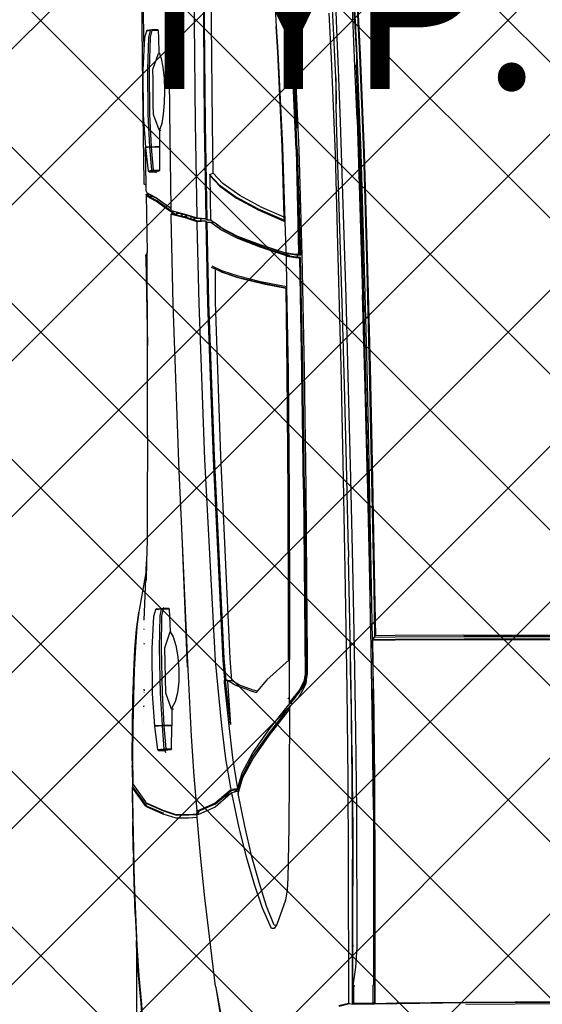
# Model space of a CAD drawing. Units: inches. Extents: x 2167 to 2589, y 1680 to 2489.
# Tile 7 of 38: x 2251 to 2275, y 1727 to 1771. Entities that reach past the tile are written whole.
import ezdxf

# ---------------------------------------------------------------- set-up
doc = ezdxf.new("R2010")
doc.units = ezdxf.units.IN
doc.header["$MEASUREMENT"] = 0
doc.layers.get('0').update_dxf_attribs({"color": 250})
for name, color, linetype, lineweight in [('A-ANNO-DIMS', 2, 'Continuous', 18), ('C-PRKG-VEHS', 8, 'Continuous', 13), ('L-PVMT-PATT', 252, 'Continuous', 13)]:
    doc.layers.add(name, color=color, linetype=linetype, lineweight=lineweight)
doc.layers.add('Edges', color=250, linetype='Continuous')
doc.styles.get("Standard").update_dxf_attribs({"font": 'arial.ttf'})
doc.dimstyles.get("Standard").update_dxf_attribs({"dimtxt": 7, "dimasz": 0.18, "dimexe": 0.18, "dimexo": 0.0625, "dimgap": 0.09, "dimtad": 0, "dimtih": 1, "dimtoh": 1, "dimdec": 1, "dimzin": 0, "dimdsep": 46, "dimlunit": 3, "dimtxsty": 'Standard', "dimcen": 0.09, "dimadec": 0, "dimazin": 0, "dimtfac": 1, "dimtdec": 1, "dimtofl": 0, "dimtmove": 0, "dimatfit": 3, "dimfxl": 1, "dimtolj": 1, "dimtzin": 0, "dimarcsym": 0})

# ---------------------------------------------------------------- blocks, each defined once
blk = doc.blocks.new('Nissan Qashqai pl')
at = {"layer": 'Edges'}
for p, q in [((10.4706, 11.5566), (10.4706, 12.2875)), ((10.4726, 11.5567), (10.4726, 12.2875)), ((10.4764, 11.5569), (10.4764, 12.2872)), ((10.4776, 11.5567), (10.4776, 12.2874)), ((11.056, 11.559), (11.0551, 11.7239)), ((11.0566, 11.5593), (11.0557, 11.724)), ((11.0586, 11.7244), (11.0595, 11.5599)), ((10.4706, 11.5566), (10.4711, 11.4469)), ((10.4731, 11.4469), (10.4726, 11.5567)), ((10.4769, 11.4474), (10.4764, 11.5569)), ((10.4781, 11.4469), (10.4776, 11.5567)), ((11.0572, 11.4499), (11.056, 11.559)), ((11.0579, 11.4504), (11.0566, 11.5593)), ((10.4711, 11.4469), (10.4715, 11.416)), ((10.4735, 11.414), (10.4731, 11.4469)), ((10.4773, 11.4146), (10.4769, 11.4474)), ((10.4785, 11.4111), (10.4781, 11.4469)), ((11.0579, 11.4146), (11.0572, 11.4499)), ((11.0585, 11.4142), (11.0579, 11.4504)), ((10.0431, 11.4075), (9.8673, 11.4031)), ((9.8673, 11.4012), (10.043, 11.4055)), ((10.2215, 11.406), (10.0429, 11.4021)), ((10.2216, 11.4037), (10.0429, 11.3998)), ((10.043, 11.4055), (10.2218, 11.4094)), ((10.2218, 11.4114), (10.0431, 11.4075)), ((10.3564, 11.406), (10.2175, 11.4028)), ((10.3945, 11.4094), (10.2215, 11.406)), ((10.3947, 11.4071), (10.2216, 11.4037)), ((10.3947, 11.4148), (10.2218, 11.4114)), ((10.2218, 11.4094), (10.3947, 11.4128)), ((10.4416, 11.4077), (10.3564, 11.406)), ((10.4773, 11.4107), (10.3945, 11.4094)), ((10.4715, 11.416), (10.3947, 11.4148)), ((10.3947, 11.4128), (10.4735, 11.414)), ((10.4416, 11.4078), (10.3947, 11.4071)), ((10.4519, 11.4079), (10.4416, 11.4077)), ((10.4519, 11.4079), (10.4416, 11.4078)), ((10.4416, 11.4077), (10.4416, 11.4078)), ((10.4524, 11.408), (10.4519, 11.4079)), ((10.4519, 11.4079), (10.4519, 11.4079)), ((10.4524, 11.4079), (10.4519, 11.4079)), ((10.4524, 11.4079), (10.4524, 11.408)), ((10.4533, 11.408), (10.4524, 11.408)), ((10.4533, 11.4079), (10.4524, 11.4079)), ((10.4638, 11.4081), (10.4533, 11.4079)), ((10.4638, 11.4081), (10.4533, 11.408)), ((10.4533, 11.4079), (10.4533, 11.408)), ((10.4914, 11.4087), (10.4638, 11.4081)), ((10.4773, 11.4107), (10.4735, 11.414)), ((10.4773, 11.4146), (10.4773, 11.4107)), ((10.4773, 11.4107), (10.5561, 11.4119)), ((10.4773, 11.4107), (10.4785, 11.4111)), ((10.5563, 11.4123), (10.4785, 11.4111)), ((10.6223, 11.4109), (10.4914, 11.4087)), ((10.6996, 11.4134), (10.5561, 11.4119)), ((10.5563, 11.4123), (10.6999, 11.4138)), ((10.7493, 11.4125), (10.6223, 11.4109)), ((10.7722, 11.4138), (10.6996, 11.4134)), ((10.6999, 11.4138), (10.7722, 11.4142)), ((10.7493, 11.4125), (11.0294, 11.4126)), ((10.7722, 11.4142), (10.7889, 11.4143)), ((10.7722, 11.4142), (10.7722, 11.4138)), ((10.7889, 11.4139), (10.7722, 11.4138)), ((10.7889, 11.4139), (10.7889, 11.4143)), ((10.7889, 11.4143), (10.7923, 11.4143)), ((10.7923, 11.4139), (10.7889, 11.4139)), ((10.7923, 11.4139), (10.7923, 11.4143)), ((10.7923, 11.4143), (10.7933, 11.4143)), ((10.7933, 11.4139), (10.7923, 11.4139)), ((10.7933, 11.4143), (10.827, 11.4145)), ((10.7933, 11.4139), (10.7933, 11.4143)), ((10.8267, 11.4141), (10.7933, 11.4139)), ((10.8267, 11.4141), (11.0585, 11.4142)), ((10.827, 11.4145), (11.0579, 11.4146)), ((11.0294, 11.4118), (11.0281, 11.4118)), ((11.0294, 11.4125), (11.0294, 11.4126)), ((11.0295, 11.4116), (11.0294, 11.4118)), ((11.0568, 11.4118), (11.0294, 11.4118)), ((11.0585, 11.4142), (11.0568, 11.4118)), ((11.0574, 11.3804), (11.0568, 11.4118)), ((11.0585, 11.4142), (11.0579, 11.4146)), ((11.0592, 11.3789), (11.0585, 11.4142)), ((9.5443, 11.3919), (9.4706, 11.388)), ((9.4709, 11.3861), (9.5446, 11.39)), ((9.701, 11.3983), (9.5443, 11.3919)), ((9.5446, 11.39), (9.7011, 11.3963)), ((9.7014, 11.3929), (9.5454, 11.3866)), ((9.7014, 11.3906), (9.5695, 11.3853)), ((9.6472, 11.3861), (9.9278, 11.3949)), ((9.6714, 11.3874), (9.8565, 11.3931)), ((9.8673, 11.4031), (9.701, 11.3983)), ((9.7011, 11.3963), (9.8673, 11.4012)), ((9.8673, 11.3977), (9.7014, 11.3929)), ((9.8673, 11.3954), (9.7014, 11.3906)), ((9.8565, 11.3931), (9.9794, 11.3967)), ((10.0429, 11.4021), (9.8673, 11.3977)), ((10.0429, 11.3998), (9.8673, 11.3954)), ((10.0747, 11.3991), (9.9278, 11.3949)), ((9.9794, 11.3967), (10.0965, 11.3998)), ((10.2043, 11.4025), (10.0747, 11.3991)), ((10.0965, 11.3998), (10.0998, 11.3999)), ((10.0998, 11.3999), (10.2043, 11.4025)), ((10.2175, 11.4028), (10.2043, 11.4025)), ((9.5105, 11.3805), (9.4694, 11.3788)), ((9.5454, 11.3866), (9.472, 11.3828)), ((9.472, 11.3812), (9.5454, 11.3851)), ((9.5755, 11.3834), (9.5105, 11.3805)), ((9.5454, 11.3851), (9.5695, 11.3853)), ((9.5454, 11.3848), (9.5454, 11.3851)), ((9.5695, 11.3853), (9.5609, 11.3849)), ((9.5695, 11.3853), (9.5786, 11.3853)), ((9.6472, 11.3861), (9.5755, 11.3834)), ((9.5786, 11.3853), (9.6206, 11.3861)), ((9.6206, 11.3861), (9.6714, 11.3874)), ((9.9312, 11.3681), (10.0776, 11.3722)), ((10.0776, 11.3722), (10.2201, 11.3759)), ((10.2201, 11.3759), (10.3586, 11.3791)), ((10.3353, 11.3725), (10.2203, 11.3699)), ((10.3353, 11.3725), (10.346, 11.3727)), ((10.4477, 11.3747), (10.346, 11.3727)), ((10.3586, 11.3791), (10.4931, 11.3817)), ((10.4537, 11.3749), (10.4477, 11.3747)), ((10.4537, 11.3749), (10.4538, 11.3749)), ((10.4681, 11.3752), (10.4538, 11.3749)), ((10.4676, 11.3751), (10.4538, 11.3749)), ((10.5576, 11.3766), (10.4676, 11.3751)), ((10.5566, 11.3765), (10.4676, 11.3751)), ((10.4676, 11.3751), (10.4676, 11.3751)), ((10.5866, 11.3772), (10.4681, 11.3752)), ((10.4931, 11.3817), (10.6237, 11.3839)), ((10.5566, 11.3765), (10.7, 11.378)), ((10.6649, 11.3783), (10.5576, 11.3766)), ((10.6649, 11.3783), (10.5866, 11.3772)), ((10.6237, 11.3839), (10.7502, 11.3855)), ((10.6908, 11.3785), (10.6649, 11.3783)), ((10.6649, 11.3783), (10.6772, 11.3784)), ((10.6966, 11.3787), (10.6772, 11.3784)), ((10.6772, 11.3784), (10.6908, 11.3785)), ((10.6991, 11.3786), (10.6908, 11.3785)), ((10.7144, 11.3788), (10.6966, 11.3787)), ((10.6999, 11.3786), (10.6991, 11.3786)), ((10.6999, 11.3786), (10.7808, 11.3793)), ((10.7144, 11.3788), (10.6999, 11.3786)), ((10.7, 11.378), (10.8279, 11.3787)), ((10.8279, 11.3727), (10.7004, 11.372)), ((10.7239, 11.3789), (10.7144, 11.3788)), ((10.7248, 11.3789), (10.7239, 11.3789)), ((10.7808, 11.3793), (10.7248, 11.3789)), ((10.7502, 11.3855), (10.968, 11.3857)), ((10.7808, 11.3793), (10.8711, 11.3796)), ((10.9431, 11.3796), (10.8279, 11.3787)), ((10.8279, 11.3787), (11.0552, 11.3789)), ((10.9614, 11.3788), (10.8279, 11.3787)), ((11.0544, 11.3728), (10.8279, 11.3727)), ((10.896, 11.3796), (10.8711, 11.3796)), ((10.9097, 11.3796), (10.896, 11.3796)), ((10.9431, 11.3796), (10.9097, 11.3796)), ((10.9478, 11.3796), (10.9431, 11.3796)), ((10.9491, 11.3796), (10.9478, 11.3796)), ((10.9668, 11.3796), (10.9491, 11.3796)), ((10.9614, 11.3788), (10.9668, 11.3796)), ((10.9711, 11.3788), (10.9614, 11.3788)), ((10.9668, 11.3796), (10.967, 11.3796)), ((10.9765, 11.3796), (10.967, 11.3796)), ((10.968, 11.3857), (11, 11.3837)), ((10.9765, 11.3796), (10.9711, 11.3788)), ((10.9766, 11.3788), (10.9711, 11.3788)), ((10.9765, 11.3796), (10.9766, 11.3788)), ((10.9825, 11.3796), (10.9765, 11.3796)), ((11.0592, 11.3789), (10.9766, 11.3788)), ((11.0301, 11.3796), (10.9825, 11.3796)), ((11, 11.3837), (11.0301, 11.3796)), ((11.0287, 11.3804), (11.0301, 11.3804)), ((11.0301, 11.3803), (11.0292, 11.3802)), ((11.03, 11.3822), (11.03, 11.3824)), ((11.0301, 11.3803), (11.0301, 11.3804)), ((11.0301, 11.3804), (11.0554, 11.3804)), ((11.0554, 11.3804), (11.0301, 11.3803)), ((11.0301, 11.3796), (11.0301, 11.3803)), ((11.0575, 11.3728), (11.0544, 11.3728)), ((11.0554, 11.3804), (11.0574, 11.3804)), ((11.0592, 11.3789), (11.0574, 11.3804)), ((11.0582, 11.3742), (11.0575, 11.3728)), ((11.0581, 11.3704), (11.0575, 11.3728)), ((11.0582, 11.3742), (11.0592, 11.3789)), ((11.0624, 11.3576), (11.0582, 11.3742)), ((9.5168, 11.3539), (9.5812, 11.3568)), ((9.5812, 11.3568), (9.6514, 11.3592)), ((9.9583, 11.363), (9.651, 11.3536)), ((9.6514, 11.3592), (9.9312, 11.3681)), ((10.0423, 11.3607), (9.8673, 11.3563)), ((10.091, 11.3666), (9.9583, 11.363)), ((10.2211, 11.3646), (10.0423, 11.3607)), ((10.2191, 11.3699), (10.091, 11.3666)), ((10.2202, 11.3699), (10.2191, 11.3699)), ((10.2202, 11.3699), (10.2203, 11.3699)), ((10.3955, 11.368), (10.2211, 11.3646)), ((10.5572, 11.3704), (10.3955, 11.368)), ((10.7004, 11.372), (10.5572, 11.3704)), ((11.0614, 11.3569), (11.0581, 11.3704)), ((9.514, 11.3492), (9.4605, 11.3465)), ((9.4761, 11.3522), (9.5168, 11.3539)), ((9.5503, 11.3455), (9.4782, 11.3418)), ((9.5811, 11.3522), (9.514, 11.3492)), ((9.7029, 11.3516), (9.5503, 11.3455)), ((9.5811, 11.3522), (9.6231, 11.3531)), ((9.594, 11.3527), (9.5811, 11.3522)), ((9.6231, 11.3531), (9.594, 11.3527)), ((9.651, 11.3536), (9.6231, 11.3531)), ((9.8673, 11.3563), (9.7029, 11.3516)), ((9.6953, 11.2892), (9.863, 11.2944)), ((9.6954, 11.2907), (9.8641, 11.2959)), ((9.696, 11.2932), (9.8644, 11.2982)), ((9.7669, 11.2945), (9.7832, 11.2951)), ((9.8629, 11.2925), (9.863, 11.2944)), ((9.8641, 11.2959), (9.863, 11.2944)), ((9.8638, 11.2934), (9.8641, 11.2959)), ((9.8644, 11.2982), (10.0472, 11.3018)), ((9.8681, 11.2959), (9.8678, 11.2935)), ((10.0476, 11.2996), (9.8681, 11.2959)), ((9.8681, 11.2959), (9.869, 11.2946)), ((9.869, 11.2946), (9.8689, 11.2927)), ((10.0477, 11.2982), (9.869, 11.2946)), ((10.0472, 11.3018), (10.2357, 11.3043)), ((10.2367, 11.3022), (10.0476, 11.2996)), ((10.2369, 11.3008), (10.0477, 11.2982)), ((10.2357, 11.3043), (10.53, 11.3068)), ((10.2367, 11.3022), (10.5351, 11.305)), ((10.2369, 11.3008), (10.5348, 11.3036)), ((10.4153, 11.3058), (10.2954, 11.3046)), ((10.4153, 11.3058), (10.4174, 11.3058)), ((10.4174, 11.3058), (10.4181, 11.3058)), ((10.4181, 11.3058), (10.4182, 11.3058)), ((10.4182, 11.3058), (10.53, 11.3068)), ((10.53, 11.3068), (10.5301, 11.3068)), ((10.5301, 11.3068), (10.5323, 11.3065)), ((10.5323, 11.3065), (10.5419, 11.3051)), ((10.5422, 11.3021), (10.5348, 11.3036)), ((10.5424, 11.3035), (10.5351, 11.305)), ((10.5366, 11.3048), (10.536, 11.305)), ((10.5379, 11.3052), (10.5381, 11.305)), ((10.5419, 11.3051), (10.5463, 11.3031)), ((10.5419, 11.3051), (10.5479, 11.3042)), ((10.5522, 11.2977), (10.5422, 11.3021)), ((10.5472, 11.3014), (10.5424, 11.3035)), ((10.5463, 11.3031), (10.5551, 11.2984)), ((10.5546, 11.2982), (10.5472, 11.3014)), ((10.5479, 11.3042), (10.5589, 11.2991)), ((10.5598, 11.2935), (10.5522, 11.2977)), ((10.5583, 11.296), (10.5546, 11.2982)), ((10.5551, 11.2984), (10.5583, 11.296)), ((10.5612, 11.2944), (10.5583, 11.296)), ((10.5589, 11.2991), (10.57, 11.2925)), ((10.5683, 11.2885), (10.5612, 11.2944)), ((9.5437, 11.2822), (9.4735, 11.2779)), ((9.5438, 11.2836), (9.4736, 11.2793)), ((9.4739, 11.282), (9.5443, 11.2863)), ((9.491, 11.2819), (9.5434, 11.2852)), ((9.6953, 11.2892), (9.5437, 11.2822)), ((9.6954, 11.2907), (9.5438, 11.2836)), ((9.5443, 11.2863), (9.696, 11.2932)), ((9.5717, 11.2865), (9.6618, 11.2907)), ((9.6953, 11.2892), (9.8598, 11.2925)), ((9.8652, 11.2788), (9.8516, 11.2363)), ((9.8629, 11.2925), (9.8598, 11.2925)), ((9.8605, 11.2746), (9.8626, 11.2878)), ((9.8615, 11.2754), (9.8635, 11.2886)), ((9.8626, 11.2878), (9.8627, 11.2909)), ((9.8627, 11.2909), (9.8629, 11.2925)), ((9.8627, 11.2909), (9.8637, 11.291)), ((9.8635, 11.2886), (9.8637, 11.291)), ((9.8637, 11.291), (9.8638, 11.2934)), ((9.8637, 11.291), (9.8643, 11.291)), ((9.8643, 11.291), (9.8677, 11.291)), ((9.8652, 11.2738), (9.8652, 11.2788)), ((9.8675, 11.2887), (9.8655, 11.2754)), ((9.8686, 11.2879), (9.8665, 11.2747)), ((9.8677, 11.291), (9.8675, 11.2887)), ((9.8678, 11.2935), (9.8677, 11.291)), ((9.8689, 11.2927), (9.8686, 11.2879)), ((10.2453, 11.2777), (10.4289, 11.2783)), ((10.4289, 11.2783), (10.5092, 11.2783)), ((10.5099, 11.2768), (10.5092, 11.2783)), ((10.5092, 11.2783), (10.5094, 11.2783)), ((10.5094, 11.2783), (10.51, 11.2776)), ((10.5783, 11.2783), (10.5094, 11.2783)), ((10.5764, 11.28), (10.5598, 11.2935)), ((10.5683, 11.2885), (10.573, 11.285)), ((10.575, 11.2829), (10.5683, 11.2885)), ((10.57, 11.2925), (10.5811, 11.2822)), ((10.573, 11.285), (10.5769, 11.2818)), ((10.5776, 11.2808), (10.575, 11.2829)), ((10.5783, 11.2783), (10.5764, 11.28)), ((10.5796, 11.2787), (10.5776, 11.2808)), ((10.5776, 11.2808), (10.5783, 11.2783)), ((10.5796, 11.2787), (10.5783, 11.2783)), ((10.5796, 11.2824), (10.5796, 11.2787)), ((10.6215, 11.2456), (10.5796, 11.2787)), ((10.5811, 11.2822), (10.5821, 11.2808)), ((10.5811, 11.2822), (10.5834, 11.28)), ((10.5821, 11.2808), (10.5834, 11.2793)), ((10.5825, 11.2806), (10.5834, 11.2793)), ((10.5834, 11.28), (10.5851, 11.2783)), ((10.5834, 11.2793), (10.5835, 11.2793)), ((10.5835, 11.2793), (10.584, 11.2787)), ((10.584, 11.2789), (10.584, 11.2793)), ((10.584, 11.2787), (10.584, 11.2789)), ((10.584, 11.2787), (10.6261, 11.2458)), ((10.584, 11.2787), (10.5851, 11.2783)), ((10.5843, 11.2787), (10.584, 11.2787)), ((10.5847, 11.2787), (10.5843, 11.2787)), ((10.5851, 11.2783), (10.5892, 11.2783)), ((10.6306, 11.2459), (10.5892, 11.2783)), ((10.5892, 11.2783), (10.6988, 11.2779)), ((10.6988, 11.2779), (10.7769, 11.2774)), ((9.5403, 11.26), (9.6913, 11.2674)), ((9.6912, 11.2667), (9.5404, 11.2598)), ((9.8039, 11.27), (9.6912, 11.2667)), ((9.6913, 11.2674), (9.8099, 11.2711)), ((9.8039, 11.27), (9.7884, 11.2343)), ((9.7905, 11.2283), (9.8087, 11.2702)), ((9.7925, 11.2294), (9.8107, 11.2711)), ((9.8087, 11.2702), (9.8039, 11.27)), ((9.8099, 11.2711), (9.8087, 11.2702)), ((9.8099, 11.2711), (9.8107, 11.2711)), ((9.8107, 11.2711), (9.8573, 11.2726)), ((9.8475, 11.2312), (9.8611, 11.2734)), ((9.8652, 11.2738), (9.8516, 11.2313)), ((9.8573, 11.2726), (9.8603, 11.2727)), ((9.8603, 11.2727), (9.8605, 11.2746)), ((9.8611, 11.2734), (9.8603, 11.2727)), ((9.8612, 11.2735), (9.8611, 11.2734)), ((9.8612, 11.2735), (9.8615, 11.2754)), ((9.8655, 11.2754), (9.8652, 11.2738)), ((9.8652, 11.2735), (9.8665, 11.2747)), ((9.8652, 11.2738), (9.8652, 11.2738)), ((9.8652, 11.2738), (9.8652, 11.2735)), ((9.8652, 11.2735), (9.8664, 11.2728)), ((9.8665, 11.2747), (9.8664, 11.2728)), ((9.8664, 11.2728), (9.9149, 11.2736)), ((9.9149, 11.2736), (9.9066, 11.2322)), ((9.9169, 11.2728), (9.9086, 11.2313)), ((9.9177, 11.2728), (9.9106, 11.2373)), ((9.9149, 11.2736), (10.0505, 11.276)), ((9.9177, 11.2728), (9.9169, 11.2728)), ((10.0501, 11.2747), (9.9177, 11.2728)), ((10.2453, 11.2762), (10.0501, 11.2747)), ((10.0505, 11.276), (10.2453, 11.2777)), ((10.4292, 11.2767), (10.2453, 11.2762)), ((10.5099, 11.2768), (10.4292, 11.2767)), ((10.51, 11.2776), (10.5099, 11.2768)), ((10.51, 11.2776), (10.5419, 11.2423)), ((10.5705, 11.2771), (10.5709, 11.2767)), ((10.5709, 11.2767), (10.5719, 11.2759)), ((10.7769, 11.2774), (10.858, 11.2759)), ((10.858, 11.2759), (10.8766, 11.2745)), ((10.8766, 11.2745), (10.8932, 11.2722)), ((10.8932, 11.2722), (10.932, 11.258)), ((9.471, 11.2554), (9.4997, 11.2573)), ((9.4997, 11.2573), (9.5403, 11.26)), ((9.5404, 11.2598), (9.4997, 11.2573)), ((10.933, 11.2541), (10.9026, 11.2417)), ((10.9384, 11.2497), (10.9059, 11.2355)), ((10.932, 11.258), (10.9335, 11.257)), ((10.9335, 11.257), (10.933, 11.2541)), ((10.9335, 11.257), (10.9386, 11.2537)), ((10.9386, 11.2537), (10.9384, 11.2497)), ((9.7884, 11.2343), (9.7692, 11.1989)), ((9.8338, 11.1956), (9.8475, 11.2312)), ((9.8516, 11.2363), (9.8378, 11.2007)), ((9.8516, 11.2313), (9.8378, 11.1957)), ((9.9066, 11.2322), (9.8978, 11.197)), ((9.9086, 11.2313), (9.8998, 11.196)), ((9.9106, 11.2373), (9.9018, 11.2021)), ((10.5419, 11.2423), (10.56, 11.2265)), ((10.6583, 11.2197), (10.6215, 11.2456)), ((10.6261, 11.2458), (10.6627, 11.22)), ((10.6671, 11.2203), (10.6306, 11.2459)), ((10.9026, 11.2417), (10.8653, 11.2297)), ((10.9059, 11.2355), (10.8682, 11.2226)), ((9.7713, 11.1929), (9.7905, 11.2283)), ((9.7733, 11.194), (9.7925, 11.2294)), ((10.5584, 11.2206), (10.5502, 11.1986)), ((10.56, 11.2265), (10.5584, 11.2206)), ((10.5584, 11.2136), (10.5617, 11.2251)), ((10.56, 11.2265), (10.5617, 11.2251)), ((10.69, 11.2028), (10.6583, 11.2197)), ((10.6627, 11.22), (10.6943, 11.2032)), ((10.6976, 11.2041), (10.6671, 11.2203)), ((10.8239, 11.2181), (10.7754, 11.2071)), ((10.8653, 11.2297), (10.8239, 11.2181)), ((10.8682, 11.2226), (10.8264, 11.21)), ((9.8378, 11.2007), (9.8241, 11.1736)), ((9.9018, 11.2021), (9.8931, 11.1752)), ((10.5584, 11.2136), (10.5502, 11.1916)), ((10.7155, 11.1952), (10.69, 11.2028)), ((10.6943, 11.2032), (10.7155, 11.1969)), ((10.7228, 11.1965), (10.6976, 11.2041)), ((10.7754, 11.2071), (10.7228, 11.1965)), ((10.8264, 11.21), (10.7776, 11.1982)), ((9.7692, 11.1989), (9.7499, 11.1721)), ((9.7519, 11.1661), (9.7713, 11.1929)), ((9.754, 11.1672), (9.7733, 11.194)), ((9.8201, 11.1685), (9.8338, 11.1956)), ((9.8378, 11.1957), (9.8241, 11.1686)), ((9.8978, 11.197), (9.8891, 11.1701)), ((9.8911, 11.1693), (9.8998, 11.196)), ((10.543, 11.1865), (10.5079, 11.1835)), ((10.5502, 11.1986), (10.543, 11.1865)), ((10.5502, 11.1916), (10.543, 11.1795)), ((10.543, 11.1795), (10.543, 11.1865)), ((10.5439, 11.1796), (10.613, 11.1841)), ((10.613, 11.1841), (10.547, 11.1767)), ((10.6144, 11.1813), (10.6664, 11.1875)), ((10.6664, 11.1875), (10.7155, 11.1952)), ((10.7137, 11.1846), (10.6678, 11.177)), ((10.7165, 11.1851), (10.7137, 11.1846)), ((10.7155, 11.1957), (10.7155, 11.1969)), ((10.7155, 11.1969), (10.7192, 11.1957)), ((10.7209, 11.1902), (10.7155, 11.1957)), ((10.7155, 11.1952), (10.7155, 11.1957)), ((10.7186, 11.1848), (10.7155, 11.1952)), ((10.7155, 11.1952), (10.7165, 11.1851)), ((10.7177, 11.1838), (10.7165, 11.1851)), ((10.7387, 11.1593), (10.7177, 11.1838)), ((10.7312, 11.1701), (10.7186, 11.1848)), ((10.7192, 11.1957), (10.7228, 11.1965)), ((10.7192, 11.1957), (10.7209, 11.1902)), ((10.7209, 11.1902), (10.7221, 11.1861)), ((10.7221, 11.1861), (10.7222, 11.1859)), ((10.7222, 11.186), (10.7221, 11.1861)), ((10.7247, 11.1867), (10.7222, 11.186)), ((10.7222, 11.186), (10.7222, 11.1859)), ((10.7222, 11.1859), (10.7232, 11.1848)), ((10.7222, 11.1859), (10.7224, 11.1855)), ((10.7224, 11.1855), (10.7312, 11.1701)), ((10.7232, 11.1848), (10.7228, 11.1859)), ((10.7232, 11.1848), (10.7449, 11.1598)), ((10.7776, 11.1982), (10.7247, 11.1867)), ((10.7257, 11.1853), (10.7256, 11.1854)), ((11.0357, 11.1613), (11.1598, 11.1847)), ((9.7499, 11.1721), (9.7337, 11.1566)), ((9.8241, 11.1686), (9.8119, 11.1529)), ((9.8241, 11.1736), (9.8147, 11.1616)), ((9.8147, 11.1616), (9.8201, 11.1685)), ((9.8891, 11.1701), (9.8818, 11.1551)), ((9.8911, 11.1691), (9.8867, 11.16)), ((9.8931, 11.1751), (9.8911, 11.1693)), ((9.8911, 11.1693), (9.8911, 11.1691)), ((9.8931, 11.1751), (9.8931, 11.1752)), ((10.1849, 11.1687), (9.9393, 11.1602)), ((10.5079, 11.1835), (10.1849, 11.1687)), ((10.5079, 11.1739), (10.1849, 11.1585)), ((10.1894, 11.1563), (10.5109, 11.1721)), ((10.543, 11.1771), (10.5079, 11.1739)), ((10.5109, 11.1721), (10.5417, 11.1748)), ((10.6152, 11.1702), (10.5113, 11.1603)), ((10.543, 11.1771), (10.5417, 11.1748)), ((10.5417, 11.1748), (10.5427, 11.1739)), ((10.5436, 11.1754), (10.5427, 11.1739)), ((10.5427, 11.1739), (10.5458, 11.1742)), ((10.5439, 11.1796), (10.543, 11.1795)), ((10.543, 11.1795), (10.543, 11.1771)), ((10.544, 11.1763), (10.543, 11.1771)), ((10.544, 11.1763), (10.5436, 11.1754)), ((10.547, 11.1767), (10.544, 11.1763)), ((10.5458, 11.1742), (10.6144, 11.1813)), ((10.6678, 11.177), (10.6152, 11.1702)), ((10.7397, 11.1602), (10.7312, 11.1701)), ((11.0492, 11.1635), (11.1336, 11.1772)), ((9.4936, 11.1538), (9.3225, 11.1531)), ((9.6552, 11.1554), (9.4936, 11.1538)), ((9.7337, 11.1566), (9.6552, 11.1554)), ((9.7357, 11.1507), (9.7337, 11.1566)), ((9.7357, 11.1507), (9.7519, 11.1661)), ((9.7378, 11.1517), (9.754, 11.1672)), ((9.8078, 11.1528), (9.7378, 11.1517)), ((9.8078, 11.1528), (9.8119, 11.1579)), ((9.8078, 11.1471), (9.8078, 11.1528)), ((9.8147, 11.1616), (9.8119, 11.1579)), ((9.8119, 11.1579), (9.8119, 11.1529)), ((9.8119, 11.1529), (9.8119, 11.1472)), ((9.8147, 11.1616), (9.8147, 11.1616)), ((9.8867, 11.16), (9.8838, 11.1541)), ((9.9393, 11.1602), (9.8867, 11.16)), ((10.1849, 11.1585), (9.9393, 11.1497)), ((9.9411, 11.1475), (10.1894, 11.1563)), ((10.5113, 11.1603), (10.19, 11.1433)), ((10.7501, 11.1327), (10.7387, 11.1593)), ((10.7507, 11.1344), (10.7397, 11.1602)), ((10.7449, 11.1598), (10.7563, 11.1333)), ((11.0304, 11.1603), (10.8896, 11.1434)), ((11.0304, 11.1603), (11.0357, 11.1613)), ((11.0357, 11.1613), (11.0491, 11.1635)), ((11.0492, 11.1635), (11.0491, 11.1635)), ((9.3198, 11.1403), (9.4922, 11.1409)), ((9.4936, 11.1428), (9.3225, 11.1421)), ((9.4922, 11.1409), (9.654, 11.1423)), ((9.6552, 11.1445), (9.4936, 11.1428)), ((9.654, 11.1423), (9.8061, 11.1447)), ((9.8078, 11.1471), (9.6552, 11.1445)), ((9.7357, 11.1507), (9.7378, 11.1517)), ((9.8061, 11.1447), (9.8051, 11.1309)), ((9.8055, 11.1298), (9.8058, 11.1369)), ((9.8058, 11.1369), (9.8061, 11.1447)), ((9.8098, 11.1369), (9.8058, 11.1369)), ((9.8061, 11.1447), (9.8078, 11.1471)), ((9.8098, 11.1369), (9.8096, 11.13)), ((9.8101, 11.1449), (9.8098, 11.1369)), ((9.8101, 11.1449), (9.9411, 11.1475)), ((9.8119, 11.1472), (9.8101, 11.1449)), ((9.8101, 11.1449), (9.8112, 11.1311)), ((9.9393, 11.1497), (9.8119, 11.1472)), ((10.19, 11.1433), (9.9414, 11.1341)), ((10.8218, 11.1365), (10.7615, 11.1311)), ((10.8896, 11.1434), (10.8218, 11.1365)), ((9.4919, 11.1269), (9.3194, 11.1262)), ((9.6538, 11.1284), (9.4919, 11.1269)), ((9.802, 11.1309), (9.6538, 11.1284)), ((9.7992, 11.1133), (9.8044, 11.129)), ((9.803, 11.1212), (9.8014, 11.1176)), ((9.8014, 11.1176), (9.8026, 11.1212)), ((9.8051, 11.1309), (9.802, 11.1309)), ((9.8026, 11.1212), (9.8041, 11.1256)), ((9.803, 11.1212), (9.8026, 11.1212)), ((9.8067, 11.1213), (9.803, 11.1212)), ((9.8041, 11.1256), (9.8045, 11.1268)), ((9.8041, 11.1256), (9.8081, 11.1256)), ((9.8044, 11.129), (9.8051, 11.1309)), ((9.8067, 11.1213), (9.8044, 11.1142)), ((9.8045, 11.1268), (9.8046, 11.1271)), ((9.8045, 11.1268), (9.8085, 11.1268)), ((9.8046, 11.1271), (9.8055, 11.1298)), ((9.8086, 11.1271), (9.8046, 11.1271)), ((9.8106, 11.1292), (9.8054, 11.1135)), ((9.8081, 11.1256), (9.8067, 11.1213)), ((9.8085, 11.1268), (9.8081, 11.1256)), ((9.8086, 11.1271), (9.8085, 11.1268)), ((9.8096, 11.13), (9.8086, 11.1271)), ((9.8112, 11.1311), (9.8106, 11.1292)), ((9.8143, 11.1312), (9.8112, 11.1311)), ((9.9414, 11.1341), (9.8143, 11.1312)), ((10.5147, 11.1156), (10.6318, 11.1213)), ((10.6318, 11.1213), (10.6955, 11.1257)), ((10.6955, 11.1257), (10.7509, 11.1302)), ((10.7507, 11.1309), (10.7501, 11.1327)), ((10.7511, 11.1335), (10.7507, 11.1344)), ((10.7507, 11.1344), (10.7524, 11.1335)), ((10.751, 11.131), (10.7507, 11.1309)), ((10.7509, 11.1302), (10.7507, 11.1309)), ((10.7522, 11.1311), (10.7509, 11.1302)), ((10.7516, 11.131), (10.7509, 11.1302)), ((10.7519, 11.1314), (10.7511, 11.1335)), ((10.7519, 11.1314), (10.7516, 11.131)), ((10.7522, 11.1311), (10.7516, 11.131)), ((10.7526, 11.1318), (10.7519, 11.1314)), ((10.7553, 11.1307), (10.7522, 11.1311)), ((10.7524, 11.1335), (10.7526, 11.1318)), ((10.7524, 11.1335), (10.7556, 11.1319)), ((10.7532, 11.1321), (10.7526, 11.1318)), ((10.7526, 11.1318), (10.7526, 11.1314)), ((10.7556, 11.1319), (10.7532, 11.1321)), ((10.7563, 11.1169), (10.7553, 11.1307)), ((10.7556, 11.1319), (10.7561, 11.1317)), ((10.7563, 11.1319), (10.7561, 11.1319)), ((10.7563, 11.1315), (10.7561, 11.1317)), ((10.7561, 11.1317), (10.7563, 11.1317)), ((10.7563, 11.1333), (10.7569, 11.1317)), ((10.7563, 11.1317), (10.7563, 11.1319)), ((10.7563, 11.1317), (10.7569, 11.1317)), ((10.7569, 11.1316), (10.7563, 11.1317)), ((10.7563, 11.1315), (10.7563, 11.1317)), ((10.7572, 11.1178), (10.7563, 11.1315)), ((10.7573, 11.1307), (10.7563, 11.1315)), ((10.7569, 11.1317), (10.7569, 11.1316)), ((10.7569, 11.1316), (10.7573, 11.1307)), ((10.7604, 11.131), (10.7573, 11.1307)), ((10.7615, 11.1311), (10.7604, 11.131)), ((10.7615, 11.1311), (10.7623, 11.1173)), ((9.7937, 11.0918), (9.7992, 11.1133)), ((9.7987, 11.1053), (9.7977, 11.1033)), ((9.7978, 11.1044), (9.7987, 11.108)), ((9.7987, 11.1053), (9.7978, 11.1044)), ((9.7987, 11.108), (9.8002, 11.1141)), ((9.7992, 11.1065), (9.7987, 11.108)), ((9.7992, 11.1065), (9.7987, 11.1053)), ((9.8027, 11.1078), (9.7992, 11.1065)), ((9.8054, 11.1135), (9.7999, 11.0919)), ((9.8002, 11.1141), (9.8008, 11.1157)), ((9.8027, 11.1078), (9.8003, 11.0983)), ((9.8008, 11.1157), (9.8014, 11.1176)), ((9.8014, 11.1139), (9.8008, 11.1157)), ((9.8043, 11.1139), (9.8014, 11.1139)), ((9.8031, 11.1093), (9.8014, 11.1139)), ((9.8031, 11.1093), (9.8027, 11.1078)), ((9.8043, 11.1139), (9.8031, 11.1093)), ((9.8044, 11.1142), (9.8043, 11.1139)), ((10.2081, 11.1017), (10.312, 11.1064)), ((10.312, 11.1064), (10.5147, 11.1156)), ((10.312, 11.1064), (10.5214, 11.1149)), ((10.7565, 11.0969), (10.7563, 11.1169)), ((10.7575, 11.0979), (10.7572, 11.1178)), ((10.7623, 11.1173), (10.7626, 11.0974)), ((9.7965, 11.0915), (9.7894, 11.0806)), ((9.7931, 11.089), (9.7934, 11.0906)), ((9.7933, 11.0892), (9.7941, 11.0901)), ((9.7934, 11.0906), (9.7937, 11.0918)), ((9.7934, 11.0906), (9.7938, 11.0904)), ((9.7941, 11.0901), (9.7943, 11.0907)), ((9.7964, 11.0988), (9.7943, 11.0907)), ((9.7955, 11.0925), (9.7943, 11.0907)), ((9.7963, 11.0918), (9.7955, 11.0925)), ((9.7992, 11.0966), (9.7963, 11.0918)), ((9.7963, 11.0918), (9.7963, 11.0918)), ((9.7964, 11.0917), (9.7963, 11.0918)), ((9.7964, 11.0988), (9.7973, 11.1023)), ((9.7964, 11.0988), (9.7992, 11.0966)), ((9.7964, 11.0917), (9.7996, 11.0966)), ((9.7964, 11.0917), (9.7964, 11.0917)), ((9.7967, 11.0915), (9.7964, 11.0917)), ((9.7965, 11.0915), (9.7967, 11.0915)), ((9.7983, 11.0901), (9.7965, 11.0915)), ((9.7967, 11.0915), (9.7986, 11.0916)), ((9.7977, 11.0907), (9.7967, 11.0915)), ((9.7973, 11.1023), (9.7977, 11.1042)), ((9.7977, 11.1033), (9.7973, 11.1023)), ((9.7973, 11.1023), (9.7977, 11.1011)), ((9.7977, 11.1042), (9.7978, 11.1044)), ((9.7977, 11.1042), (9.7977, 11.1033)), ((9.7977, 11.1011), (9.7977, 11.0998)), ((9.7977, 11.1011), (9.7985, 11.099)), ((9.7977, 11.0998), (9.7985, 11.099)), ((9.7982, 11.0902), (9.7977, 11.0907)), ((9.7986, 11.0916), (9.7982, 11.0902)), ((9.7983, 11.0901), (9.7982, 11.0902)), ((9.7986, 11.0898), (9.7983, 11.0901)), ((9.7985, 11.099), (9.7989, 11.098)), ((9.7988, 11.0925), (9.7986, 11.0916)), ((9.7986, 11.0898), (9.7993, 11.0891)), ((9.7998, 11.0964), (9.7988, 11.0925)), ((9.7989, 11.098), (9.7998, 11.0976)), ((9.7998, 11.0976), (9.7992, 11.0966)), ((9.7999, 11.0919), (9.7993, 11.0891)), ((9.8002, 11.098), (9.7996, 11.0966)), ((9.8001, 11.0974), (9.7996, 11.0966)), ((9.7996, 11.0966), (9.7998, 11.0964)), ((9.8003, 11.0983), (9.7998, 11.0976)), ((9.8001, 11.0974), (9.7998, 11.0964)), ((9.8002, 11.098), (9.8001, 11.0974)), ((9.8003, 11.0983), (9.8002, 11.098)), ((9.8024, 11.0892), (9.9426, 11.0923)), ((9.9426, 11.0923), (10.2081, 11.1017)), ((10.4653, 11.0881), (10.4652, 11.0897)), ((10.4653, 11.0881), (10.4732, 11.0925)), ((10.4732, 11.0925), (10.4871, 11.0967)), ((10.4871, 11.0967), (10.5048, 11.1002)), ((10.5048, 11.1002), (10.5246, 11.1019)), ((10.5246, 11.1019), (10.5445, 11.1017)), ((10.5445, 11.1017), (10.5625, 11.0996)), ((10.5625, 11.0996), (10.5769, 11.0957)), ((10.5867, 11.0897), (10.563, 11.0809)), ((10.5769, 11.0957), (10.5863, 11.0904)), ((10.5863, 11.0904), (10.5867, 11.0897)), ((10.5885, 11.0904), (10.5867, 11.0897)), ((10.5885, 11.0931), (10.5885, 11.0904)), ((10.5885, 11.0904), (10.6141, 11.0905)), ((10.6141, 11.0905), (10.615, 11.0905)), ((10.6142, 11.0782), (10.6141, 11.0905)), ((10.6517, 11.0902), (10.615, 11.0905)), ((10.615, 11.0905), (10.6151, 11.0782)), ((10.6518, 11.0808), (10.6517, 11.0902)), ((10.6517, 11.0902), (10.6535, 11.0895)), ((10.6535, 11.0895), (10.6543, 11.0786)), ((10.6535, 11.0895), (10.6536, 11.0803)), ((10.7497, 11.0763), (10.7565, 11.0969)), ((10.7507, 11.0773), (10.7575, 11.0979)), ((10.7626, 11.0974), (10.7559, 11.0767)), ((9.4673, 11.0852), (9.6358, 11.0866)), ((9.5503, 11.0736), (9.5641, 11.076)), ((9.5641, 11.076), (9.5818, 11.0782)), ((9.5818, 11.0782), (9.6016, 11.0791)), ((9.6016, 11.0791), (9.6215, 11.0782)), ((9.6215, 11.0782), (9.6395, 11.0766)), ((9.6358, 11.0866), (9.7887, 11.0889)), ((9.6395, 11.0766), (9.654, 11.0744)), ((9.654, 11.0744), (9.6633, 11.0715)), ((9.7728, 11.066), (9.7832, 11.0805)), ((9.7738, 11.067), (9.7842, 11.0814)), ((9.7883, 11.0815), (9.7778, 11.0671)), ((9.7894, 11.0806), (9.7788, 11.0661)), ((9.7832, 11.0805), (9.7887, 11.0889)), ((9.7842, 11.0814), (9.7891, 11.0889)), ((9.7933, 11.0892), (9.7883, 11.0815)), ((9.7887, 11.0889), (9.7891, 11.0889)), ((9.7891, 11.0889), (9.79, 11.0889)), ((9.79, 11.0889), (9.7931, 11.089)), ((9.7931, 11.089), (9.7933, 11.0892)), ((9.7993, 11.0891), (9.8024, 11.0892)), ((10.4263, 11.0777), (10.4274, 11.0767)), ((10.4274, 11.0767), (10.4275, 11.0856)), ((10.4274, 11.0762), (10.4274, 11.0767)), ((10.4282, 11.0666), (10.4274, 11.0762)), ((10.4275, 11.0856), (10.4293, 11.0863)), ((10.4293, 11.0863), (10.4291, 11.0765)), ((10.4291, 11.0765), (10.4398, 11.0741)), ((10.4398, 11.0718), (10.4291, 11.0741)), ((10.4291, 11.0741), (10.4299, 11.0644)), ((10.4293, 11.0863), (10.4398, 11.0868)), ((10.4398, 11.0868), (10.4653, 11.0878)), ((10.4398, 11.0741), (10.4909, 11.0734)), ((10.4653, 11.0877), (10.4653, 11.0881)), ((10.4653, 11.0878), (10.4653, 11.0881)), ((10.4653, 11.0881), (10.4653, 11.0881)), ((10.4653, 11.0877), (10.4653, 11.0878)), ((10.4908, 11.0793), (10.4653, 11.0877)), ((10.563, 11.0809), (10.4908, 11.0793)), ((10.4909, 11.0734), (10.563, 11.075)), ((10.563, 11.075), (10.6142, 11.0779)), ((10.6142, 11.0756), (10.5631, 11.0727)), ((10.6142, 11.0779), (10.6142, 11.0782)), ((10.6142, 11.0765), (10.6142, 11.0779)), ((10.615, 11.0765), (10.6142, 11.0765)), ((10.6142, 11.0756), (10.6142, 11.0765)), ((10.615, 11.0639), (10.6142, 11.0756)), ((10.6151, 11.0765), (10.615, 11.0765)), ((10.615, 11.0765), (10.6151, 11.0639)), ((10.6151, 11.078), (10.6518, 11.0808)), ((10.6518, 11.0784), (10.6151, 11.0756)), ((10.6151, 11.0782), (10.6151, 11.078)), ((10.6151, 11.078), (10.6151, 11.0765)), ((10.6151, 11.0765), (10.6151, 11.0756)), ((10.6151, 11.0756), (10.616, 11.0629)), ((10.6518, 11.0784), (10.6518, 11.0808)), ((10.6518, 11.0808), (10.6536, 11.0803)), ((10.6536, 11.0803), (10.6518, 11.0784)), ((10.6526, 11.0674), (10.6518, 11.0784)), ((10.6536, 11.0803), (10.6537, 11.0783)), ((10.6543, 11.0786), (10.6537, 11.0783)), ((10.6537, 11.0783), (10.6543, 11.0693)), ((10.6578, 11.0814), (10.6543, 11.0786)), ((10.6543, 11.0693), (10.6543, 11.0786)), ((10.7385, 11.051), (10.7497, 11.0763)), ((10.7396, 11.0519), (10.7507, 11.0773)), ((10.7549, 11.0776), (10.743, 11.0503)), ((10.7559, 11.0767), (10.7448, 11.0511)), ((9.5037, 11.0635), (9.5045, 11.0628)), ((9.5044, 11.0586), (9.5045, 11.0628)), ((9.5052, 11.0524), (9.5044, 11.0586)), ((9.5045, 11.0683), (9.5063, 11.0687)), ((9.5045, 11.0628), (9.5045, 11.0683)), ((9.5063, 11.0687), (9.5061, 11.0586)), ((9.5061, 11.0586), (9.5167, 11.0559)), ((9.5063, 11.0687), (9.5168, 11.0691)), ((9.5168, 11.0691), (9.5423, 11.0696)), ((9.5422, 11.0706), (9.5422, 11.0716)), ((9.5422, 11.0706), (9.5424, 11.0707)), ((9.5423, 11.0696), (9.5422, 11.0706)), ((9.5426, 11.0695), (9.5423, 11.0696)), ((9.5424, 11.0707), (9.5503, 11.0736)), ((9.5426, 11.0695), (9.5424, 11.0707)), ((9.5667, 11.0609), (9.5426, 11.0695)), ((9.5678, 11.0604), (9.5667, 11.0609)), ((9.5846, 11.0606), (9.5678, 11.0604)), ((9.6236, 11.0609), (9.5846, 11.0606)), ((9.64, 11.0611), (9.6236, 11.0609)), ((9.6413, 11.0616), (9.64, 11.0611)), ((9.6645, 11.0705), (9.6413, 11.0616)), ((9.6633, 11.0715), (9.6645, 11.0705)), ((9.6655, 11.0708), (9.6645, 11.0705)), ((9.6655, 11.0728), (9.6655, 11.0708)), ((9.6655, 11.0708), (9.6911, 11.0709)), ((9.6911, 11.0709), (9.692, 11.0709)), ((9.6911, 11.0645), (9.6911, 11.0709)), ((9.6912, 11.0631), (9.6911, 11.0645)), ((9.692, 11.0631), (9.6912, 11.0631)), ((9.6912, 11.0577), (9.6912, 11.0631)), ((9.692, 11.0709), (9.692, 11.0645)), ((9.692, 11.0709), (9.7287, 11.0708)), ((9.692, 11.0645), (9.692, 11.0631)), ((9.692, 11.0631), (9.6921, 11.0578)), ((9.6921, 11.0578), (9.7288, 11.0609)), ((9.7288, 11.0588), (9.6922, 11.0556)), ((9.7287, 11.0708), (9.7305, 11.0704)), ((9.7288, 11.0609), (9.7287, 11.0708)), ((9.7288, 11.0588), (9.7288, 11.0609)), ((9.7288, 11.0609), (9.7306, 11.0607)), ((9.7306, 11.0607), (9.7288, 11.0588)), ((9.7296, 11.0527), (9.7288, 11.0588)), ((9.7305, 11.0704), (9.7313, 11.0644)), ((9.7305, 11.0704), (9.7306, 11.0607)), ((9.7306, 11.0607), (9.7314, 11.0547)), ((9.733, 11.066), (9.7313, 11.0644)), ((9.7314, 11.0547), (9.7313, 11.0644)), ((9.7674, 11.0557), (9.7728, 11.066)), ((9.7684, 11.0567), (9.7717, 11.0631)), ((9.7717, 11.0631), (9.7707, 11.0593)), ((9.7707, 11.0593), (9.7709, 11.0549)), ((9.7717, 11.0631), (9.7738, 11.067)), ((9.7778, 11.0671), (9.7724, 11.0568)), ((9.7788, 11.0661), (9.7734, 11.0558)), ((10.4282, 11.0666), (10.4299, 11.0644)), ((10.4299, 11.0644), (10.4406, 11.0612)), ((10.4909, 11.0711), (10.4398, 11.0718)), ((10.4406, 11.0612), (10.4919, 11.0584)), ((10.5631, 11.0727), (10.4909, 11.0711)), ((10.4919, 11.0584), (10.564, 11.0591)), ((10.564, 11.0591), (10.6151, 11.0628)), ((10.6151, 11.0639), (10.615, 11.0639)), ((10.6151, 11.0628), (10.615, 11.0639)), ((10.6151, 11.0639), (10.6151, 11.0628)), ((10.616, 11.0629), (10.6526, 11.0674)), ((10.6526, 11.0674), (10.6543, 11.0693)), ((9.2517, 11.0411), (9.5372, 11.0459)), ((9.641, 11.045), (9.351, 11.0411)), ((9.5052, 11.0524), (9.5069, 11.0501)), ((9.5168, 11.0537), (9.5061, 11.0564)), ((9.5061, 11.0564), (9.5069, 11.0501)), ((9.5069, 11.0501), (9.5176, 11.0469)), ((9.5167, 11.0559), (9.5679, 11.0543)), ((9.5679, 11.0521), (9.5168, 11.0537)), ((9.5176, 11.0469), (9.5372, 11.0459)), ((9.5372, 11.0459), (9.5689, 11.0442)), ((9.5679, 11.0543), (9.64, 11.0549)), ((9.6401, 11.0528), (9.5679, 11.0521)), ((9.5689, 11.0442), (9.641, 11.045)), ((9.64, 11.0549), (9.6912, 11.0577)), ((9.6913, 11.0556), (9.6401, 11.0528)), ((9.641, 11.045), (9.6921, 11.0485)), ((9.7466, 11.0464), (9.641, 11.045)), ((9.6913, 11.0556), (9.6912, 11.0577)), ((9.692, 11.0499), (9.6913, 11.0556)), ((9.6922, 11.0499), (9.692, 11.0499)), ((9.6921, 11.0485), (9.692, 11.0499)), ((9.6922, 11.0556), (9.6921, 11.0578)), ((9.6922, 11.0499), (9.6921, 11.0485)), ((9.7526, 11.0495), (9.6921, 11.0485)), ((9.6922, 11.0556), (9.693, 11.0486)), ((9.6922, 11.0556), (9.6922, 11.0499)), ((9.693, 11.0486), (9.7296, 11.0527)), ((9.7296, 11.0527), (9.7314, 11.0547)), ((9.7511, 11.0463), (9.7466, 11.0464)), ((9.7526, 11.0495), (9.7511, 11.0463)), ((9.7623, 11.0497), (9.7526, 11.0495)), ((9.7623, 11.0497), (9.7643, 11.0504)), ((9.7643, 11.0504), (9.7652, 11.0514)), ((9.7643, 11.0504), (9.7648, 11.0513)), ((9.7648, 11.0513), (9.7664, 11.054)), ((9.7648, 11.0513), (9.7648, 11.0513)), ((9.7652, 11.0514), (9.7665, 11.0535)), ((9.7664, 11.054), (9.7674, 11.0557)), ((9.7665, 11.0537), (9.7664, 11.054)), ((9.7665, 11.0535), (9.7676, 11.0553)), ((9.7667, 11.0508), (9.7665, 11.0535)), ((9.7676, 11.0511), (9.7667, 11.0508)), ((9.7677, 11.0498), (9.7667, 11.0508)), ((9.7673, 11.0545), (9.7676, 11.0553)), ((9.7673, 11.0543), (9.7673, 11.0545)), ((9.7676, 11.0511), (9.7673, 11.0543)), ((9.7676, 11.0553), (9.7684, 11.0567)), ((9.7676, 11.0555), (9.7678, 11.056)), ((9.769, 11.0516), (9.7676, 11.0511)), ((9.7677, 11.0498), (9.8598, 11.0514)), ((9.77, 11.0506), (9.7677, 11.0498)), ((9.7677, 11.0498), (9.7677, 11.0498)), ((9.7712, 11.055), (9.769, 11.0516)), ((9.7734, 11.0558), (9.77, 11.0506)), ((9.7709, 11.0549), (9.7712, 11.055)), ((9.7724, 11.0568), (9.7712, 11.055)), ((9.8598, 11.0514), (9.8614, 11.0504)), ((9.8643, 11.0514), (9.8598, 11.0514)), ((9.8614, 11.0504), (9.8647, 11.0485)), ((10.0085, 11.0519), (9.8643, 11.0514)), ((9.8647, 11.0485), (9.869, 11.0488)), ((9.869, 11.0488), (10.0085, 11.0519)), ((10.0124, 11.0519), (10.0085, 11.0519)), ((10.1513, 11.0517), (10.0124, 11.0519)), ((10.1513, 11.0517), (10.2677, 11.0512)), ((10.2677, 11.0512), (10.3189, 11.0511)), ((10.3189, 11.0511), (10.3537, 11.0503)), ((10.3537, 11.0503), (10.3832, 11.0496)), ((10.3679, 11.0497), (10.3537, 11.0503)), ((10.3679, 11.0497), (10.4275, 11.0391)), ((10.4468, 11.0466), (10.3679, 11.0497)), ((10.4502, 11.0466), (10.4503, 11.0465)), ((10.4613, 11.0464), (10.4603, 11.0465)), ((10.4838, 11.0465), (10.4852, 11.046)), ((10.5565, 11.0456), (10.5591, 11.0464)), ((10.5615, 11.0464), (10.5617, 11.0457)), ((10.583, 11.0457), (10.5835, 11.0461)), ((10.5836, 11.0461), (10.5832, 11.0457)), ((10.5847, 11.0461), (10.5841, 11.0457)), ((10.5873, 11.0461), (10.5873, 11.0461)), ((10.6087, 11.0458), (10.6087, 11.0458)), ((10.7087, 11.0289), (10.7363, 11.0483)), ((10.7424, 11.0499), (10.7125, 11.0285)), ((10.7429, 11.0485), (10.7148, 11.0284)), ((10.7363, 11.0483), (10.7376, 11.0492)), ((10.7387, 11.0502), (10.7376, 11.0492)), ((10.7376, 11.0492), (10.7378, 11.0495)), ((10.7378, 11.0495), (10.7385, 11.051)), ((10.7378, 11.0495), (10.7379, 11.0496)), ((10.7387, 11.0502), (10.7396, 11.0519)), ((10.7424, 11.0499), (10.743, 11.0503)), ((10.7429, 11.0488), (10.7432, 11.0488)), ((10.7432, 11.0488), (10.7429, 11.0485)), ((10.744, 11.0494), (10.7432, 11.0488)), ((10.7448, 11.0511), (10.744, 11.0494)), ((11.0798, 11.0434), (11.0576, 11.0416)), ((11.059, 11.0419), (11.0768, 11.0434)), ((10.4275, 11.0391), (10.4304, 11.0385)), ((10.4304, 11.0385), (10.4339, 11.0381)), ((10.4345, 11.0379), (10.4339, 11.0381)), ((10.4339, 11.0381), (10.4573, 11.0349)), ((10.4613, 11.0343), (10.4345, 11.0379)), ((10.4573, 11.0349), (10.4889, 11.0323)), ((10.4926, 11.0317), (10.4613, 11.0343)), ((10.4889, 11.0323), (10.526, 11.0304)), ((10.5294, 11.0298), (10.4926, 11.0317)), ((10.526, 11.0304), (10.569, 11.0291)), ((10.5719, 11.0285), (10.5294, 11.0298)), ((10.569, 11.0291), (10.5919, 11.0287)), ((10.6176, 11.0277), (10.5719, 11.0285)), ((10.5919, 11.0287), (10.5936, 11.0286)), ((10.5936, 11.0286), (10.6151, 11.0283)), ((10.6151, 11.0283), (10.6644, 11.028)), ((10.6651, 11.0274), (10.6176, 11.0277)), ((10.6644, 11.028), (10.7078, 11.0282)), ((10.677, 11.0275), (10.6651, 11.0274)), ((10.7082, 11.0285), (10.6729, 11.0284)), ((10.68, 11.0274), (10.677, 11.0275)), ((10.6809, 11.0274), (10.68, 11.0274)), ((10.6809, 11.0274), (10.7128, 11.0275)), ((10.7078, 11.0282), (10.7083, 11.0285)), ((10.7082, 11.0285), (10.7078, 11.0282)), ((10.7085, 11.0289), (10.7082, 11.0285)), ((10.7083, 11.0285), (10.7082, 11.0285)), ((10.7083, 11.0285), (10.7087, 11.0289)), ((10.7125, 11.0285), (10.7083, 11.0285)), ((10.7146, 11.0286), (10.7125, 11.0285)), ((10.7125, 11.0285), (10.7139, 11.0278)), ((10.7134, 11.0275), (10.7128, 11.0275)), ((10.7625, 11.0281), (10.7134, 11.0275)), ((10.724, 11.0275), (10.7134, 11.0275)), ((10.7148, 11.0284), (10.7139, 11.0278)), ((10.7628, 11.0283), (10.7139, 11.0278)), ((10.724, 11.0275), (10.7685, 11.0281)), ((10.7628, 11.0281), (10.7625, 11.0281)), ((10.7628, 11.0283), (10.8131, 11.0292)), ((10.7628, 11.0281), (10.8131, 11.029)), ((10.7688, 11.0281), (10.7685, 11.0281)), ((10.8131, 11.029), (10.7688, 11.0281)), ((10.8131, 11.0292), (10.8644, 11.0306)), ((10.8132, 11.029), (10.8131, 11.029)), ((10.8132, 11.029), (10.8139, 11.029)), ((10.8142, 11.029), (10.8139, 11.029)), ((10.8142, 11.029), (10.8241, 11.0293)), ((10.8142, 11.029), (10.8142, 11.029)), ((10.8242, 11.0293), (10.8241, 11.0293)), ((10.8246, 11.0293), (10.8242, 11.0293)), ((10.8642, 11.0304), (10.8246, 11.0293)), ((10.9152, 11.0321), (10.8642, 11.0304)), ((10.8642, 11.0305), (10.8759, 11.031)), ((10.8644, 11.0306), (10.8759, 11.031)), ((10.8759, 11.031), (10.9158, 11.0324)), ((10.9152, 11.0321), (10.9577, 11.0341)), ((10.9158, 11.0324), (10.9657, 11.0347)), ((10.9649, 11.0344), (10.9577, 11.0341)), ((10.9577, 11.0341), (11.1283, 11.0341)), ((11.0127, 11.0375), (10.9649, 11.0344)), ((10.9657, 11.0347), (11.0138, 11.0377)), ((11.0576, 11.0416), (11.0127, 11.0375)), ((11.0138, 11.0377), (11.059, 11.0419))]:
    blk.add_line(p, q, dxfattribs=at)
blk = doc.blocks.new('car')
blk.add_blockref('Nissan Qashqai pl', (-9.7433, -11.9151))
blk = doc.blocks.new('carr')
blk.add_blockref('car', (0.5124, -0.007))
blk = doc.blocks.new('*D45')
at = {"layer": 'A-ANNO-DIMS', "color": 0, "lineweight": -2, "transparency": 16777216}
for p, q in [((2251.156, 1833.955), (2232.359, 1833.955)), ((2232.539, 1833.775), (2232.539, 1775.399)), ((2232.539, 1709.605), (2232.539, 1767.981)), ((2251.156, 1709.425), (2232.359, 1709.425))]:
    blk.add_line(p, q, dxfattribs=at)
at = {"layer": 'A-ANNO-DIMS', "color": 0, "transparency": 16777216}
for points in [[(2232.509, 1833.775), (2232.569, 1833.775), (2232.539, 1833.955)], [(2232.509, 1709.605), (2232.569, 1709.605), (2232.539, 1709.425)]]:
    blk.add_solid(points, dxfattribs=at)
at = {"layer": 'Defpoints', "color": 0, "transparency": 16777216}
for p in [(2251.218, 1833.955), (2232.539, 1709.425), (2251.218, 1709.425)]:
    blk.add_point(p, dxfattribs=at)
at = {"layer": 'A-ANNO-DIMS', "color": 0, "transparency": 16777216, "insert": (2232.539, 1771.69), "char_height": 7, "attachment_point": 5}
blk.add_mtext('\\A1;CAR 10\'-4 1/2" TYP.', dxfattribs=at)

msp = doc.modelspace()

# ---------------------------------------------------------------- hatches: boundary and pattern name
at = {"layer": 'L-PVMT-PATT'}
h = msp.add_hatch(dxfattribs=at)
h.set_pattern_fill('ANSI37', color=256, scale=40)
h.paths.add_polyline_path([(2417.548, 1783.695), (2417.548, 1846.042), (2239.361, 1846.042), (2239.361, 1687.695), (2369.843, 1687.695), (2369.843, 1696.695), (2375.607, 1696.695), (2416.107, 1696.695), (2417.548, 1696.695)])

# ---------------------------------------------------------------- block references
at = {"layer": 'C-PRKG-VEHS', "xscale": 28.42784210623918, "yscale": 28.42784210623918, "zscale": 28.42784210623918, "rotation": 270}
msp.add_blockref('carr', (2281.736, 1778.659), dxfattribs=at)

# ---------------------------------------------------------------- dimensions: what is measured, and where the dimension line sits
at = {"layer": 'A-ANNO-DIMS'}
dim = msp.add_linear_dim(base=(2232.539, 1709.425), p1=(2251.218, 1833.955), p2=(2251.218, 1709.425), angle=270, text='CAR <> TYP.', dimstyle='Standard', override={"dimdec": 1, "dimlfac": 1, "dimrnd": 0, "dimzin": 1, "dimdsep": 46, "dimlunit": 4, "dimfrac": 2}, dxfattribs=at)
dim.commit()
dim.dimension.update_dxf_attribs({"geometry": '*D45', "text_midpoint": (2232.539, 1771.69)})

doc.saveas('drawing.dxf')
